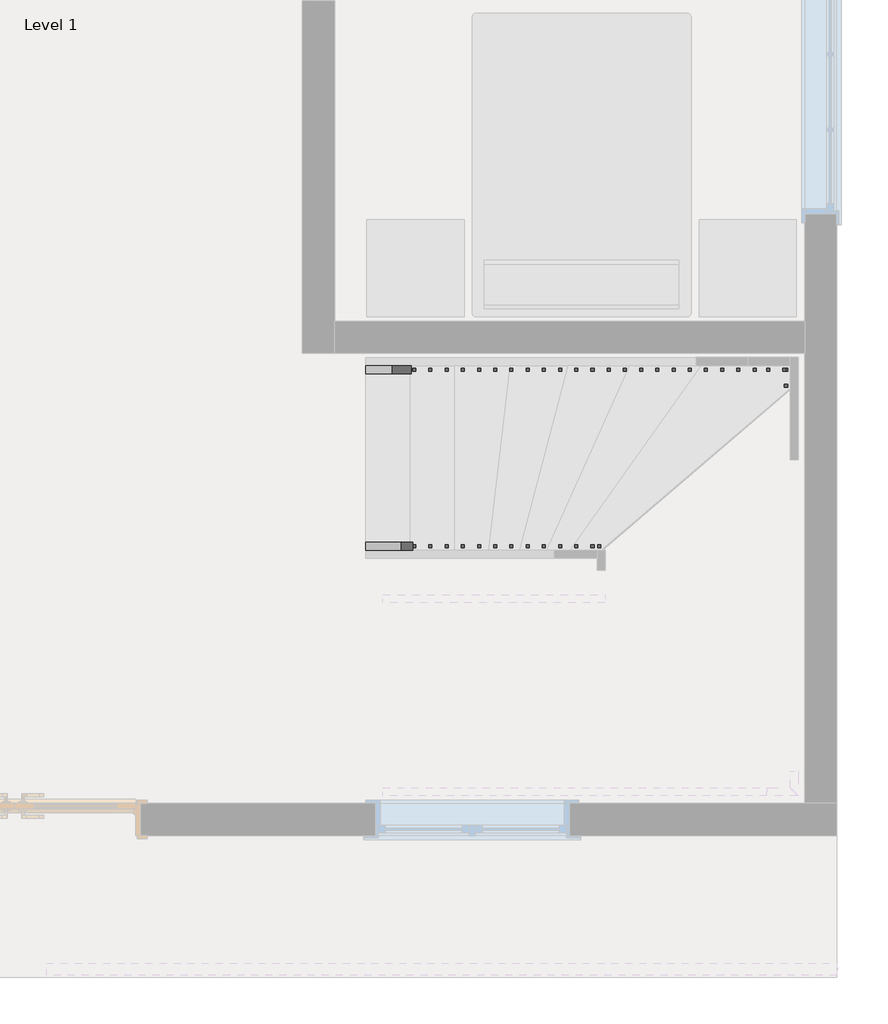
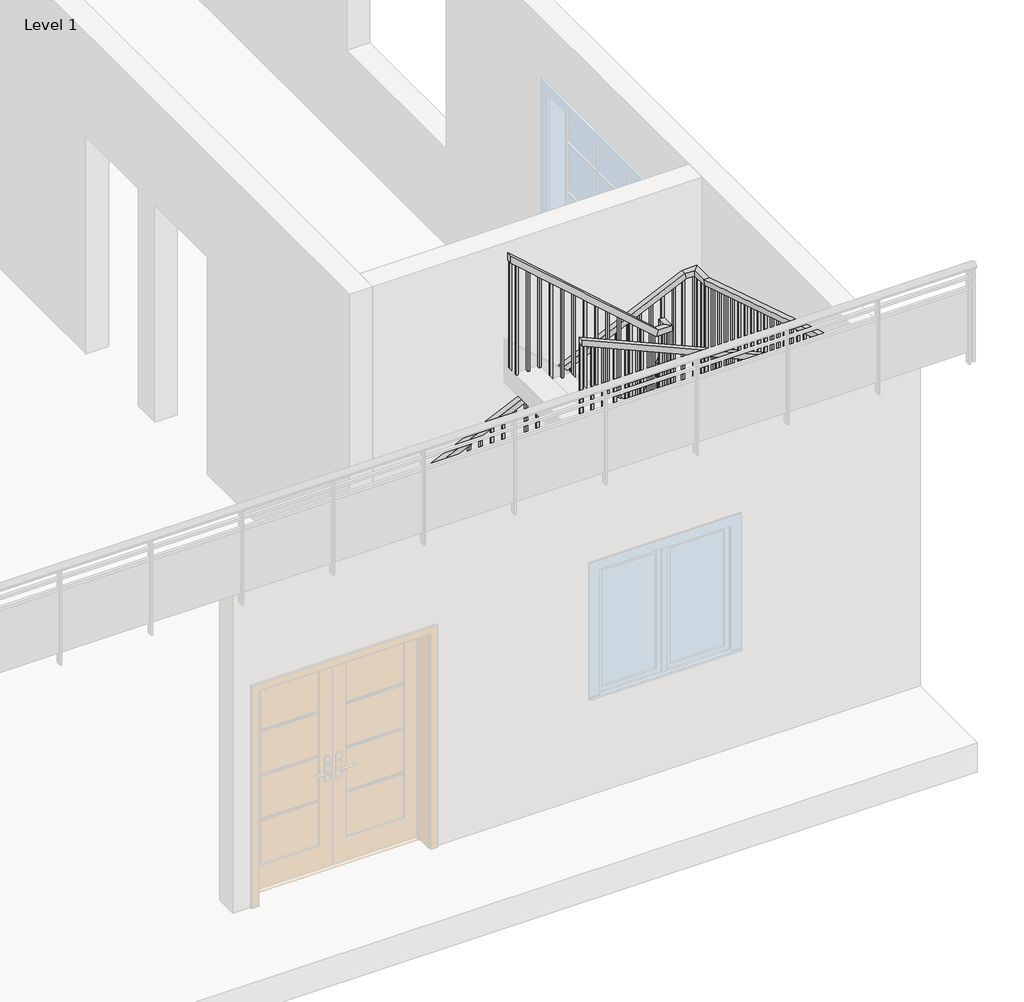
# One storey, part 3 of 4: 2 railings.
"""IFC4 building model written with IfcOpenShell, lengths in millimetres."""

from ifc_helpers import new_model, si_unit, frame, origin, place, context, project, spatial, polyline, outline, extrude, faceted_brep, element, save

model = new_model("IFC4")

# Units and contexts
model_context = context("Model", 3, world=origin())
ifc_project = project(units=[si_unit("LENGTHUNIT", "METRE", prefix="MILLI")], contexts=[model_context])

# Site, building, storey
site = spatial("IfcSite", under=ifc_project)
building = spatial("IfcBuilding", under=site)
storey = spatial("IfcBuildingStorey", under=building, Name="Level 1", Elevation=0.0)

# Railings
placement = place(None, origin())
element("IfcRailing", 1, ObjectType="Handrail - Rectangular", at=placement, inside=storey, context=model_context, shape_type="SolidModel", body=[
    faceted_brep([(-5318.5510787, 1481.9501077, 1007.9778391), (-5318.5510787, 1481.9501077, 940.4028685), (-5318.5510787, 1431.1501077, 940.4028685), (-5318.5510787, 1431.1501077, 1007.9778391), (-3853.6690894, 1481.9501077, 2292.967851), (-3834.5457095, 1481.9501077, 2242.167851), (-3834.5457095, 1431.1501077, 2242.167851), (-3853.6690894, 1431.1501077, 2292.967851), (-3764.9367614, 1481.9501077, 2292.967851), (-3764.9367614, 1431.1501077, 2292.967851), (-3764.9367614, 1431.1501077, 2242.167851), (-3764.9367614, 1481.9501077, 2242.167851)], [[[0, 1, 2, 3]], [[1, 0, 4, 5]], [[2, 1, 5, 6]], [[3, 2, 6, 7]], [[0, 3, 7, 4]], [[8, 9, 10, 11]], [[5, 4, 8, 11]], [[6, 5, 11, 10]], [[7, 6, 10, 9]], [[4, 7, 9, 8]]]),
    faceted_brep([(-3764.9367614, 1431.1501077, 2288.9786494), (-3764.9367614, 1431.1501077, 2174.0145886), (-3815.7367614, 1431.1501077, 2174.0145886), (-3815.7367614, 1431.1501077, 2288.9786494), (-3764.9367614, 1177.1501077, 2804.6358827), (-3764.9367614, 1126.3501077, 2792.8032685), (-3815.7367614, 1126.3501077, 2792.8032685), (-3815.7367614, 1177.1501077, 2804.6358827), (-5209.7542153, 1050.1501077, 4209.1766651), (-5209.7542153, 1100.9501077, 4209.1766651), (-5209.7542153, 1100.9501077, 4141.3989335), (-5209.7542153, 1050.1501077, 4141.3989335), (-3911.1589121, 1050.1501077, 2994.4303641), (-3891.9367614, 1050.1501077, 3045.2303641), (-3911.1589121, 1100.9501077, 2994.4303641), (-3891.9367614, 1100.9501077, 3045.2303641), (-3764.9367614, 1177.1501077, 3045.2303641), (-3764.9367614, 1126.3501077, 2994.4303641), (-3815.7367614, 1126.3501077, 2994.4303641), (-3815.7367614, 1177.1501077, 3045.2303641), (-3764.9367614, 1050.1501077, 3045.2303641), (-3764.9367614, 1050.1501077, 2994.4303641), (-3815.7367614, 1100.9501077, 2994.4303641), (-3815.7367614, 1100.9501077, 3045.2303641)], [[[0, 1, 2, 3]], [[1, 0, 4, 5]], [[2, 1, 5, 6]], [[3, 2, 6, 7]], [[0, 3, 7, 4]], [[8, 9, 10, 11]], [[12, 13, 8, 11]], [[14, 12, 11, 10]], [[15, 14, 10, 9]], [[13, 15, 9, 8]], [[5, 4, 16, 17]], [[6, 5, 17, 18]], [[7, 6, 18, 19]], [[4, 7, 19, 16]], [[17, 16, 20, 21]], [[18, 17, 21, 22]], [[19, 18, 22, 23]], [[16, 19, 23, 20]], [[21, 20, 13, 12]], [[22, 21, 12, 14]], [[23, 22, 14, 15]], [[20, 23, 15, 13]]]),
    extrude(outline(polyline([(4073.5861118, -5132.976687), (4090.4117935, -5152.026687), (3048.0, -5152.026687), (3048.0, -5132.976687), (4073.5861118, -5132.976687)])), frame((0.0, 1066.0251077, 0.0), z_axis=(0.0, 1.0, 0.0), x_axis=(0.0, 0.0, 1.0)), (0.0, 0.0, 1.0), 19.05),
    extrude(outline(polyline([(3983.8491427, -5031.376687), (4000.6748244, -5050.426687), (3048.0, -5050.426687), (3048.0, -5031.376687), (3983.8491427, -5031.376687)])), frame((0.0, 1066.0251077, 0.0), z_axis=(0.0, 1.0, 0.0), x_axis=(0.0, 0.0, 1.0)), (0.0, 0.0, 1.0), 19.05),
    extrude(outline(polyline([(3894.1121735, -4929.776687), (3910.9378552, -4948.826687), (3048.0, -4948.826687), (3048.0, -4929.776687), (3894.1121735, -4929.776687)])), frame((0.0, 1066.0251077, 0.0), z_axis=(0.0, 1.0, 0.0), x_axis=(0.0, 0.0, 1.0)), (0.0, 0.0, 1.0), 19.05),
    extrude(outline(polyline([(3804.3752044, -4828.176687), (3821.2008861, -4847.226687), (2878.6666667, -4847.226687), (2878.6666667, -4828.176687), (3804.3752044, -4828.176687)])), frame((0.0, 1066.0251077, 0.0), z_axis=(0.0, 1.0, 0.0), x_axis=(0.0, 0.0, 1.0)), (0.0, 0.0, 1.0), 19.05),
    extrude(outline(polyline([(3714.6382352, -4726.576687), (3731.4639169, -4745.626687), (2878.6666667, -4745.626687), (2878.6666667, -4726.576687), (3714.6382352, -4726.576687)])), frame((0.0, 1066.0251077, 0.0), z_axis=(0.0, 1.0, 0.0), x_axis=(0.0, 0.0, 1.0)), (0.0, 0.0, 1.0), 19.05),
    extrude(outline(polyline([(3624.9012661, -4624.976687), (3641.7269478, -4644.026687), (2709.3333333, -4644.026687), (2709.3333333, -4624.976687), (3624.9012661, -4624.976687)])), frame((0.0, 1066.0251077, 0.0), z_axis=(0.0, 1.0, 0.0), x_axis=(0.0, 0.0, 1.0)), (0.0, 0.0, 1.0), 19.05),
    extrude(outline(polyline([(3535.1642969, -4523.376687), (3551.9899786, -4542.426687), (2709.3333333, -4542.426687), (2709.3333333, -4523.376687), (3535.1642969, -4523.376687)])), frame((0.0, 1066.0251077, 0.0), z_axis=(0.0, 1.0, 0.0), x_axis=(0.0, 0.0, 1.0)), (0.0, 0.0, 1.0), 19.05),
    extrude(outline(polyline([(3445.4273278, -4421.776687), (3462.2530095, -4440.826687), (2540.0, -4440.826687), (2540.0, -4421.776687), (3445.4273278, -4421.776687)])), frame((0.0, 1066.0251077, 0.0), z_axis=(0.0, 1.0, 0.0), x_axis=(0.0, 0.0, 1.0)), (0.0, 0.0, 1.0), 19.05),
    extrude(outline(polyline([(3355.6903586, -4320.176687), (3372.5160404, -4339.226687), (2540.0, -4339.226687), (2540.0, -4320.176687), (3355.6903586, -4320.176687)])), frame((0.0, 1066.0251077, 0.0), z_axis=(0.0, 1.0, 0.0), x_axis=(0.0, 0.0, 1.0)), (0.0, 0.0, 1.0), 19.05),
    extrude(outline(polyline([(3265.9533895, -4218.576687), (3282.7790712, -4237.626687), (2370.6666667, -4237.626687), (2370.6666667, -4218.576687), (3265.9533895, -4218.576687)])), frame((0.0, 1066.0251077, 0.0), z_axis=(0.0, 1.0, 0.0), x_axis=(0.0, 0.0, 1.0)), (0.0, 0.0, 1.0), 19.05),
    extrude(outline(polyline([(3176.2164204, -4116.976687), (3193.0421021, -4136.026687), (2370.6666667, -4136.026687), (2370.6666667, -4116.976687), (3176.2164204, -4116.976687)])), frame((0.0, 1066.0251077, 0.0), z_axis=(0.0, 1.0, 0.0), x_axis=(0.0, 0.0, 1.0)), (0.0, 0.0, 1.0), 19.05),
    extrude(outline(polyline([(3086.4794512, -4015.376687), (3103.3051329, -4034.426687), (2201.3333333, -4034.426687), (2201.3333333, -4015.376687), (3086.4794512, -4015.376687)])), frame((0.0, 1066.0251077, 0.0), z_axis=(0.0, 1.0, 0.0), x_axis=(0.0, 0.0, 1.0)), (0.0, 0.0, 1.0), 19.05),
    extrude(outline(polyline([(2996.7424821, -3913.776687), (3013.5681638, -3932.826687), (2032.0, -3932.826687), (2032.0, -3913.776687), (2996.7424821, -3913.776687)])), frame((0.0, 1066.0251077, 0.0), z_axis=(0.0, 1.0, 0.0), x_axis=(0.0, 0.0, 1.0)), (0.0, 0.0, 1.0), 19.05),
    extrude(outline(polyline([(1114.8601257, 2816.1296163), (1133.9101257, 2777.4553238), (1133.9101257, 1862.6666667), (1114.8601257, 1862.6666667), (1114.8601257, 2816.1296163)])), frame((-3799.8617614, 0.0, 0.0), z_axis=(1.0, 0.0, 0.0), x_axis=(0.0, 1.0, 0.0)), (0.0, 0.0, 1.0), 19.05),
    extrude(outline(polyline([(1216.4601257, 2609.866723), (1235.5101257, 2571.1924305), (1235.5101257, 1693.3333333), (1216.4601257, 1693.3333333), (1216.4601257, 2609.866723)])), frame((-3799.8617614, 0.0, 0.0), z_axis=(1.0, 0.0, 0.0), x_axis=(0.0, 1.0, 0.0)), (0.0, 0.0, 1.0), 19.05),
    extrude(outline(polyline([(1318.0601257, 2403.6038297), (1337.1101257, 2364.9295372), (1337.1101257, 1524.0), (1318.0601257, 1524.0), (1318.0601257, 2403.6038297)])), frame((-3799.8617614, 0.0, 0.0), z_axis=(1.0, 0.0, 0.0), x_axis=(0.0, 1.0, 0.0)), (0.0, 0.0, 1.0), 19.05),
    extrude(outline(polyline([(2196.48311, -3886.6260787), (2179.7725081, -3905.6760787), (1185.3333333, -3905.6760787), (1185.3333333, -3886.6260787), (2196.48311, -3886.6260787)])), frame((0.0, 1447.0251077, 0.0), z_axis=(0.0, 1.0, 0.0), x_axis=(0.0, 0.0, 1.0)), (0.0, 0.0, 1.0), 19.05),
    extrude(outline(polyline([(2107.3598999, -3988.2260787), (2090.6492981, -4007.2760787), (1185.3333333, -4007.2760787), (1185.3333333, -3988.2260787), (2107.3598999, -3988.2260787)])), frame((0.0, 1447.0251077, 0.0), z_axis=(0.0, 1.0, 0.0), x_axis=(0.0, 0.0, 1.0)), (0.0, 0.0, 1.0), 19.05),
    extrude(outline(polyline([(2018.2366899, -4089.8260787), (2001.526088, -4108.8760787), (1016.0, -4108.8760787), (1016.0, -4089.8260787), (2018.2366899, -4089.8260787)])), frame((0.0, 1447.0251077, 0.0), z_axis=(0.0, 1.0, 0.0), x_axis=(0.0, 0.0, 1.0)), (0.0, 0.0, 1.0), 19.05),
    extrude(outline(polyline([(1929.1134799, -4191.4260787), (1912.402878, -4210.4760787), (846.6666667, -4210.4760787), (846.6666667, -4191.4260787), (1929.1134799, -4191.4260787)])), frame((0.0, 1447.0251077, 0.0), z_axis=(0.0, 1.0, 0.0), x_axis=(0.0, 0.0, 1.0)), (0.0, 0.0, 1.0), 19.05),
    extrude(outline(polyline([(1839.9902698, -4293.0260787), (1823.279668, -4312.0760787), (846.6666667, -4312.0760787), (846.6666667, -4293.0260787), (1839.9902698, -4293.0260787)])), frame((0.0, 1447.0251077, 0.0), z_axis=(0.0, 1.0, 0.0), x_axis=(0.0, 0.0, 1.0)), (0.0, 0.0, 1.0), 19.05),
    extrude(outline(polyline([(1750.8670598, -4394.6260787), (1734.1564579, -4413.6760787), (677.3333333, -4413.6760787), (677.3333333, -4394.6260787), (1750.8670598, -4394.6260787)])), frame((0.0, 1447.0251077, 0.0), z_axis=(0.0, 1.0, 0.0), x_axis=(0.0, 0.0, 1.0)), (0.0, 0.0, 1.0), 19.05),
    extrude(outline(polyline([(1661.7438498, -4496.2260787), (1645.0332479, -4515.2760787), (677.3333333, -4515.2760787), (677.3333333, -4496.2260787), (1661.7438498, -4496.2260787)])), frame((0.0, 1447.0251077, 0.0), z_axis=(0.0, 1.0, 0.0), x_axis=(0.0, 0.0, 1.0)), (0.0, 0.0, 1.0), 19.05),
    extrude(outline(polyline([(1572.6206397, -4597.8260787), (1555.9100378, -4616.8760787), (508.0, -4616.8760787), (508.0, -4597.8260787), (1572.6206397, -4597.8260787)])), frame((0.0, 1447.0251077, 0.0), z_axis=(0.0, 1.0, 0.0), x_axis=(0.0, 0.0, 1.0)), (0.0, 0.0, 1.0), 19.05),
    extrude(outline(polyline([(1483.4974297, -4699.4260787), (1466.7868278, -4718.4760787), (508.0, -4718.4760787), (508.0, -4699.4260787), (1483.4974297, -4699.4260787)])), frame((0.0, 1447.0251077, 0.0), z_axis=(0.0, 1.0, 0.0), x_axis=(0.0, 0.0, 1.0)), (0.0, 0.0, 1.0), 19.05),
    extrude(outline(polyline([(1394.3742197, -4801.0260787), (1377.6636178, -4820.0760787), (338.6666667, -4820.0760787), (338.6666667, -4801.0260787), (1394.3742197, -4801.0260787)])), frame((0.0, 1447.0251077, 0.0), z_axis=(0.0, 1.0, 0.0), x_axis=(0.0, 0.0, 1.0)), (0.0, 0.0, 1.0), 19.05),
    extrude(outline(polyline([(1305.2510096, -4902.6260787), (1288.5404077, -4921.6760787), (338.6666667, -4921.6760787), (338.6666667, -4902.6260787), (1305.2510096, -4902.6260787)])), frame((0.0, 1447.0251077, 0.0), z_axis=(0.0, 1.0, 0.0), x_axis=(0.0, 0.0, 1.0)), (0.0, 0.0, 1.0), 19.05),
    extrude(outline(polyline([(1216.1277996, -5004.2260787), (1199.4171977, -5023.2760787), (338.6666667, -5023.2760787), (338.6666667, -5004.2260787), (1216.1277996, -5004.2260787)])), frame((0.0, 1447.0251077, 0.0), z_axis=(0.0, 1.0, 0.0), x_axis=(0.0, 0.0, 1.0)), (0.0, 0.0, 1.0), 19.05),
    extrude(outline(polyline([(1127.0045896, -5105.8260787), (1110.2939877, -5124.8760787), (169.3333333, -5124.8760787), (169.3333333, -5105.8260787), (1127.0045896, -5105.8260787)])), frame((0.0, 1447.0251077, 0.0), z_axis=(0.0, 1.0, 0.0), x_axis=(0.0, 0.0, 1.0)), (0.0, 0.0, 1.0), 19.05),
    extrude(outline(polyline([(1037.8813795, -5207.4260787), (1021.1707776, -5226.4760787), (169.3333333, -5226.4760787), (169.3333333, -5207.4260787), (1037.8813795, -5207.4260787)])), frame((0.0, 1447.0251077, 0.0), z_axis=(0.0, 1.0, 0.0), x_axis=(0.0, 0.0, 1.0)), (0.0, 0.0, 1.0), 19.05),
    extrude(outline(polyline([(-3812.176687, 1085.0751077), (-3812.176687, 1066.0251077), (-3831.226687, 1066.0251077), (-3831.226687, 1085.0751077), (-3812.176687, 1085.0751077)])), frame((0.0, 0.0, 2032.0), z_axis=(0.0, 0.0, 1.0), x_axis=(1.0, 0.0, 0.0)), (0.0, 0.0, 1.0), 962.4303641),
    extrude(outline(polyline([(-3799.8617614, 1085.0751077), (-3780.8117614, 1085.0751077), (-3780.8117614, 1066.0251077), (-3799.8617614, 1066.0251077), (-3799.8617614, 1085.0751077)])), frame((0.0, 0.0, 2032.0), z_axis=(0.0, 0.0, 1.0), x_axis=(1.0, 0.0, 0.0)), (0.0, 0.0, 1.0), 962.4303641),
    extrude(outline(polyline([(-3799.8617614, 1098.7207679), (-3780.8117614, 1098.7207679), (-3780.8117614, 1079.6707679), (-3799.8617614, 1079.6707679), (-3799.8617614, 1098.7207679)])), frame((0.0, 0.0, 2032.0), z_axis=(0.0, 0.0, 1.0), x_axis=(1.0, 0.0, 0.0)), (0.0, 0.0, 1.0), 962.4303641),
    extrude(outline(polyline([(1419.6601257, 2197.3409364), (1438.7101257, 2158.6666439), (1438.7101257, 1354.6666667), (1419.6601257, 1354.6666667), (1419.6601257, 2197.3409364)])), frame((-3799.8617614, 0.0, 0.0), z_axis=(1.0, 0.0, 0.0), x_axis=(0.0, 1.0, 0.0)), (0.0, 0.0, 1.0), 19.05),
    extrude(outline(polyline([(-3799.8617614, 1447.0251077), (-3799.8617614, 1466.0751077), (-3780.8117614, 1466.0751077), (-3780.8117614, 1447.0251077), (-3799.8617614, 1447.0251077)])), frame((0.0, 0.0, 1354.6666667), z_axis=(0.0, 0.0, 1.0), x_axis=(1.0, 0.0, 0.0)), (0.0, 0.0, 1.0), 887.5011843),
    extrude(outline(polyline([(2233.7481814, -3844.1440894), (2217.0375795, -3863.1940894), (1185.3333333, -3863.1940894), (1185.3333333, -3844.1440894), (2233.7481814, -3844.1440894)])), frame((0.0, 1447.0251077, 0.0), z_axis=(0.0, 1.0, 0.0), x_axis=(0.0, 0.0, 1.0)), (0.0, 0.0, 1.0), 19.05),
    extrude(outline(polyline([(4124.5732518, -5190.7042153), (4141.3989335, -5209.7542153), (3048.0, -5209.7542153), (3048.0, -5190.7042153), (4124.5732518, -5190.7042153)])), frame((0.0, 1066.0251077, 0.0), z_axis=(0.0, 1.0, 0.0), x_axis=(0.0, 0.0, 1.0)), (0.0, 0.0, 1.0), 19.05),
    extrude(outline(polyline([(957.1134704, -5299.5010787), (940.4028685, -5318.5510787), (169.3333333, -5318.5510787), (169.3333333, -5299.5010787), (957.1134704, -5299.5010787)])), frame((0.0, 1447.0251077, 0.0), z_axis=(0.0, 1.0, 0.0), x_axis=(0.0, 0.0, 1.0)), (0.0, 0.0, 1.0), 19.05),
])
element("IfcRailing", 2, ObjectType="Handrail - Rectangular", at=placement, inside=storey, context=model_context, shape_type="SolidModel", body=[
    faceted_brep([(-5318.5510787, 2589.1174997, 1123.4764008), (-5318.5510787, 2589.1174997, 1067.4781727), (-5318.5510787, 2538.3174997, 1067.4781727), (-5318.5510787, 2538.3174997, 1123.4764008), (-2794.8351304, 2589.1174997, 2294.0169189), (-2783.6276147, 2589.1174997, 2243.2169189), (-2783.6276147, 2538.3174997, 2243.2169189), (-2794.8351304, 2538.3174997, 2294.0169189), (-2657.7693695, 2589.1174997, 2294.0169189), (-2657.7693695, 2589.1174997, 2243.2169189), (-2708.5693695, 2538.3174997, 2243.2169189), (-2708.5693695, 2538.3174997, 2294.0169189), (-2657.7693695, 2398.3356848, 2294.0169189), (-2657.7693695, 2390.5672195, 2243.2169189), (-2708.5693695, 2390.5672195, 2243.2169189), (-2708.5693695, 2398.3356848, 2294.0169189), (-2657.7693695, -57.0172843, 2966.0525983), (-2657.7693695, -57.0172843, 3016.8525983), (-2770.3188697, -57.0172843, 3016.8525983), (-2780.9506148, -57.0172843, 2966.0525983), (-2708.5693695, -6.2172843, 2966.0525983), (-2780.9506148, -6.2172843, 2966.0525983), (-2708.5693695, -6.2172843, 3016.8525983), (-2770.3188697, -6.2172843, 3016.8525983), (-2657.7693695, 90.2000505, 3016.8525983), (-2657.7693695, 82.4315853, 2966.0525983), (-2708.5693695, 82.4315853, 2966.0525983), (-2708.5693695, 90.2000505, 3016.8525983), (-5209.7542153, -57.0172843, 4084.706306), (-5209.7542153, -6.2172843, 4084.706306), (-5209.7542153, -6.2172843, 4029.2522993), (-5209.7542153, -57.0172843, 4029.2522993)], [[[0, 1, 2, 3]], [[1, 0, 4, 5]], [[2, 1, 5, 6]], [[3, 2, 6, 7]], [[0, 3, 7, 4]], [[5, 4, 8, 9]], [[6, 5, 9, 10]], [[7, 6, 10, 11]], [[4, 7, 11, 8]], [[9, 8, 12, 13]], [[10, 9, 13, 14]], [[11, 10, 14, 15]], [[8, 11, 15, 12]], [[16, 17, 18, 19]], [[20, 16, 19, 21]], [[22, 20, 21, 23]], [[17, 22, 23, 18]], [[13, 12, 24, 25]], [[14, 13, 25, 26]], [[15, 14, 26, 27]], [[12, 15, 27, 24]], [[25, 24, 17, 16]], [[26, 25, 16, 20]], [[27, 26, 20, 22]], [[24, 27, 22, 17]], [[28, 29, 30, 31]], [[19, 18, 28, 31]], [[21, 19, 31, 30]], [[23, 21, 30, 29]], [[18, 23, 29, 28]]]),
    extrude(outline(polyline([(4032.9686139, -5218.2438697), (3048.0, -5218.2438697), (3048.0, -5199.1938697), (4024.6295475, -5199.1938697), (4032.9686139, -5218.2438697)])), frame((0.0, -41.1422843, 0.0), z_axis=(0.0, 1.0, 0.0), x_axis=(0.0, 0.0, 1.0)), (0.0, 0.0, 1.0), 19.05),
    extrude(outline(polyline([(3988.4935935, -5116.6438697), (3048.0, -5116.6438697), (3048.0, -5097.5938697), (3980.1545272, -5097.5938697), (3988.4935935, -5116.6438697)])), frame((0.0, -41.1422843, 0.0), z_axis=(0.0, 1.0, 0.0), x_axis=(0.0, 0.0, 1.0)), (0.0, 0.0, 1.0), 19.05),
    extrude(outline(polyline([(3944.0185731, -5015.0438697), (3048.0, -5015.0438697), (3048.0, -4995.9938697), (3935.6795068, -4995.9938697), (3944.0185731, -5015.0438697)])), frame((0.0, -41.1422843, 0.0), z_axis=(0.0, 1.0, 0.0), x_axis=(0.0, 0.0, 1.0)), (0.0, 0.0, 1.0), 19.05),
    extrude(outline(polyline([(3899.5435527, -4913.4438697), (2878.6666667, -4913.4438697), (2878.6666667, -4894.3938697), (3891.2044864, -4894.3938697), (3899.5435527, -4913.4438697)])), frame((0.0, -41.1422843, 0.0), z_axis=(0.0, 1.0, 0.0), x_axis=(0.0, 0.0, 1.0)), (0.0, 0.0, 1.0), 19.05),
    extrude(outline(polyline([(3855.0685323, -4811.8438697), (2878.6666667, -4811.8438697), (2878.6666667, -4792.7938697), (3846.729466, -4792.7938697), (3855.0685323, -4811.8438697)])), frame((0.0, -41.1422843, 0.0), z_axis=(0.0, 1.0, 0.0), x_axis=(0.0, 0.0, 1.0)), (0.0, 0.0, 1.0), 19.05),
    extrude(outline(polyline([(3810.593512, -4710.2438697), (2878.6666667, -4710.2438697), (2878.6666667, -4691.1938697), (3802.2544456, -4691.1938697), (3810.593512, -4710.2438697)])), frame((0.0, -41.1422843, 0.0), z_axis=(0.0, 1.0, 0.0), x_axis=(0.0, 0.0, 1.0)), (0.0, 0.0, 1.0), 19.05),
    extrude(outline(polyline([(3766.1184916, -4608.6438697), (2709.3333333, -4608.6438697), (2709.3333333, -4589.5938697), (3757.7794253, -4589.5938697), (3766.1184916, -4608.6438697)])), frame((0.0, -41.1422843, 0.0), z_axis=(0.0, 1.0, 0.0), x_axis=(0.0, 0.0, 1.0)), (0.0, 0.0, 1.0), 19.05),
    extrude(outline(polyline([(3721.6434712, -4507.0438697), (2709.3333333, -4507.0438697), (2709.3333333, -4487.9938697), (3713.3044049, -4487.9938697), (3721.6434712, -4507.0438697)])), frame((0.0, -41.1422843, 0.0), z_axis=(0.0, 1.0, 0.0), x_axis=(0.0, 0.0, 1.0)), (0.0, 0.0, 1.0), 19.05),
    extrude(outline(polyline([(3677.1684508, -4405.4438697), (2709.3333333, -4405.4438697), (2709.3333333, -4386.3938697), (3668.8293845, -4386.3938697), (3677.1684508, -4405.4438697)])), frame((0.0, -41.1422843, 0.0), z_axis=(0.0, 1.0, 0.0), x_axis=(0.0, 0.0, 1.0)), (0.0, 0.0, 1.0), 19.05),
    extrude(outline(polyline([(3632.6934304, -4303.8438697), (2540.0, -4303.8438697), (2540.0, -4284.7938697), (3624.3543641, -4284.7938697), (3632.6934304, -4303.8438697)])), frame((0.0, -41.1422843, 0.0), z_axis=(0.0, 1.0, 0.0), x_axis=(0.0, 0.0, 1.0)), (0.0, 0.0, 1.0), 19.05),
    extrude(outline(polyline([(3588.2184101, -4202.2438697), (2540.0, -4202.2438697), (2540.0, -4183.1938697), (3579.8793437, -4183.1938697), (3588.2184101, -4202.2438697)])), frame((0.0, -41.1422843, 0.0), z_axis=(0.0, 1.0, 0.0), x_axis=(0.0, 0.0, 1.0)), (0.0, 0.0, 1.0), 19.05),
    extrude(outline(polyline([(3543.7433897, -4100.6438697), (2540.0, -4100.6438697), (2540.0, -4081.5938697), (3535.4043233, -4081.5938697), (3543.7433897, -4100.6438697)])), frame((0.0, -41.1422843, 0.0), z_axis=(0.0, 1.0, 0.0), x_axis=(0.0, 0.0, 1.0)), (0.0, 0.0, 1.0), 19.05),
    extrude(outline(polyline([(3499.2683693, -3999.0438697), (2540.0, -3999.0438697), (2540.0, -3979.9938697), (3490.929303, -3979.9938697), (3499.2683693, -3999.0438697)])), frame((0.0, -41.1422843, 0.0), z_axis=(0.0, 1.0, 0.0), x_axis=(0.0, 0.0, 1.0)), (0.0, 0.0, 1.0), 19.05),
    extrude(outline(polyline([(3454.7933489, -3897.4438697), (2370.6666667, -3897.4438697), (2370.6666667, -3878.3938697), (3446.4542826, -3878.3938697), (3454.7933489, -3897.4438697)])), frame((0.0, -41.1422843, 0.0), z_axis=(0.0, 1.0, 0.0), x_axis=(0.0, 0.0, 1.0)), (0.0, 0.0, 1.0), 19.05),
    extrude(outline(polyline([(3410.3183285, -3795.8438697), (2370.6666667, -3795.8438697), (2370.6666667, -3776.7938697), (3401.9792622, -3776.7938697), (3410.3183285, -3795.8438697)])), frame((0.0, -41.1422843, 0.0), z_axis=(0.0, 1.0, 0.0), x_axis=(0.0, 0.0, 1.0)), (0.0, 0.0, 1.0), 19.05),
    extrude(outline(polyline([(3365.8433081, -3694.2438697), (2370.6666667, -3694.2438697), (2370.6666667, -3675.1938697), (3357.5042418, -3675.1938697), (3365.8433081, -3694.2438697)])), frame((0.0, -41.1422843, 0.0), z_axis=(0.0, 1.0, 0.0), x_axis=(0.0, 0.0, 1.0)), (0.0, 0.0, 1.0), 19.05),
    extrude(outline(polyline([(3321.3682878, -3592.6438697), (2370.6666667, -3592.6438697), (2370.6666667, -3573.5938697), (3313.0292214, -3573.5938697), (3321.3682878, -3592.6438697)])), frame((0.0, -41.1422843, 0.0), z_axis=(0.0, 1.0, 0.0), x_axis=(0.0, 0.0, 1.0)), (0.0, 0.0, 1.0), 19.05),
    extrude(outline(polyline([(3276.8932674, -3491.0438697), (2201.3333333, -3491.0438697), (2201.3333333, -3471.9938697), (3268.5542011, -3471.9938697), (3276.8932674, -3491.0438697)])), frame((0.0, -41.1422843, 0.0), z_axis=(0.0, 1.0, 0.0), x_axis=(0.0, 0.0, 1.0)), (0.0, 0.0, 1.0), 19.05),
    extrude(outline(polyline([(3232.418247, -3389.4438697), (2201.3333333, -3389.4438697), (2201.3333333, -3370.3938697), (3224.0791807, -3370.3938697), (3232.418247, -3389.4438697)])), frame((0.0, -41.1422843, 0.0), z_axis=(0.0, 1.0, 0.0), x_axis=(0.0, 0.0, 1.0)), (0.0, 0.0, 1.0), 19.05),
    extrude(outline(polyline([(3187.9432266, -3287.8438697), (2201.3333333, -3287.8438697), (2201.3333333, -3268.7938697), (3179.6041603, -3268.7938697), (3187.9432266, -3287.8438697)])), frame((0.0, -41.1422843, 0.0), z_axis=(0.0, 1.0, 0.0), x_axis=(0.0, 0.0, 1.0)), (0.0, 0.0, 1.0), 19.05),
    extrude(outline(polyline([(3143.4682062, -3186.2438697), (2201.3333333, -3186.2438697), (2201.3333333, -3167.1938697), (3135.1291399, -3167.1938697), (3143.4682062, -3186.2438697)])), frame((0.0, -41.1422843, 0.0), z_axis=(0.0, 1.0, 0.0), x_axis=(0.0, 0.0, 1.0)), (0.0, 0.0, 1.0), 19.05),
    extrude(outline(polyline([(3098.9931859, -3084.6438697), (2201.3333333, -3084.6438697), (2201.3333333, -3065.5938697), (3090.6541195, -3065.5938697), (3098.9931859, -3084.6438697)])), frame((0.0, -41.1422843, 0.0), z_axis=(0.0, 1.0, 0.0), x_axis=(0.0, 0.0, 1.0)), (0.0, 0.0, 1.0), 19.05),
    extrude(outline(polyline([(3054.5181655, -2983.0438697), (2032.0, -2983.0438697), (2032.0, -2963.9938697), (3046.1790992, -2963.9938697), (3054.5181655, -2983.0438697)])), frame((0.0, -41.1422843, 0.0), z_axis=(0.0, 1.0, 0.0), x_axis=(0.0, 0.0, 1.0)), (0.0, 0.0, 1.0), 19.05),
    extrude(outline(polyline([(3010.0431451, -2881.4438697), (2032.0, -2881.4438697), (2032.0, -2862.3938697), (3001.7040788, -2862.3938697), (3010.0431451, -2881.4438697)])), frame((0.0, -41.1422843, 0.0), z_axis=(0.0, 1.0, 0.0), x_axis=(0.0, 0.0, 1.0)), (0.0, 0.0, 1.0), 19.05),
    extrude(outline(polyline([(-2673.6443695, -1.8749495), (-2673.6443695, -20.9249495), (-2692.6943695, -20.9249495), (-2692.6943695, -1.8749495), (-2673.6443695, -1.8749495)])), frame((0.0, 0.0, 2032.0), z_axis=(0.0, 0.0, 1.0), x_axis=(1.0, 0.0, 0.0)), (0.0, 0.0, 1.0), 934.0525983),
    extrude(outline(polyline([(172.6606848, 2937.7956746), (172.6606848, 2032.0), (153.6106848, 2032.0), (153.6106848, 2943.761537), (172.6606848, 2937.7956746)])), frame((-2692.6943695, 0.0, 0.0), z_axis=(1.0, 0.0, 0.0), x_axis=(0.0, 1.0, 0.0)), (0.0, 0.0, 1.0), 19.05),
    extrude(outline(polyline([(274.2606848, 2905.9777416), (274.2606848, 2032.0), (255.2106848, 2032.0), (255.2106848, 2911.943604), (274.2606848, 2905.9777416)])), frame((-2692.6943695, 0.0, 0.0), z_axis=(1.0, 0.0, 0.0), x_axis=(0.0, 1.0, 0.0)), (0.0, 0.0, 1.0), 19.05),
    extrude(outline(polyline([(375.8606848, 2874.1598085), (375.8606848, 1862.6666667), (356.8106848, 1862.6666667), (356.8106848, 2880.125671), (375.8606848, 2874.1598085)])), frame((-2692.6943695, 0.0, 0.0), z_axis=(1.0, 0.0, 0.0), x_axis=(0.0, 1.0, 0.0)), (0.0, 0.0, 1.0), 19.05),
    extrude(outline(polyline([(477.4606848, 2842.3418755), (477.4606848, 1862.6666667), (458.4106848, 1862.6666667), (458.4106848, 2848.3077379), (477.4606848, 2842.3418755)])), frame((-2692.6943695, 0.0, 0.0), z_axis=(1.0, 0.0, 0.0), x_axis=(0.0, 1.0, 0.0)), (0.0, 0.0, 1.0), 19.05),
    extrude(outline(polyline([(579.0606848, 2810.5239425), (579.0606848, 1862.6666667), (560.0106848, 1862.6666667), (560.0106848, 2816.4898049), (579.0606848, 2810.5239425)])), frame((-2692.6943695, 0.0, 0.0), z_axis=(1.0, 0.0, 0.0), x_axis=(0.0, 1.0, 0.0)), (0.0, 0.0, 1.0), 19.05),
    extrude(outline(polyline([(680.6606848, 2778.7060094), (680.6606848, 1862.6666667), (661.6106848, 1862.6666667), (661.6106848, 2784.6718719), (680.6606848, 2778.7060094)])), frame((-2692.6943695, 0.0, 0.0), z_axis=(1.0, 0.0, 0.0), x_axis=(0.0, 1.0, 0.0)), (0.0, 0.0, 1.0), 19.05),
    extrude(outline(polyline([(782.2606848, 2746.8880764), (782.2606848, 1862.6666667), (763.2106848, 1862.6666667), (763.2106848, 2752.8539389), (782.2606848, 2746.8880764)])), frame((-2692.6943695, 0.0, 0.0), z_axis=(1.0, 0.0, 0.0), x_axis=(0.0, 1.0, 0.0)), (0.0, 0.0, 1.0), 19.05),
    extrude(outline(polyline([(883.8606848, 2715.0701434), (883.8606848, 1862.6666667), (864.8106848, 1862.6666667), (864.8106848, 2721.0360058), (883.8606848, 2715.0701434)])), frame((-2692.6943695, 0.0, 0.0), z_axis=(1.0, 0.0, 0.0), x_axis=(0.0, 1.0, 0.0)), (0.0, 0.0, 1.0), 19.05),
    extrude(outline(polyline([(985.4606848, 2683.2522104), (985.4606848, 1693.3333333), (966.4106848, 1693.3333333), (966.4106848, 2689.2180728), (985.4606848, 2683.2522104)])), frame((-2692.6943695, 0.0, 0.0), z_axis=(1.0, 0.0, 0.0), x_axis=(0.0, 1.0, 0.0)), (0.0, 0.0, 1.0), 19.05),
    extrude(outline(polyline([(1087.0606848, 2651.4342773), (1087.0606848, 1693.3333333), (1068.0106848, 1693.3333333), (1068.0106848, 2657.4001398), (1087.0606848, 2651.4342773)])), frame((-2692.6943695, 0.0, 0.0), z_axis=(1.0, 0.0, 0.0), x_axis=(0.0, 1.0, 0.0)), (0.0, 0.0, 1.0), 19.05),
    extrude(outline(polyline([(1188.6606848, 2619.6163443), (1188.6606848, 1693.3333333), (1169.6106848, 1693.3333333), (1169.6106848, 2625.5822068), (1188.6606848, 2619.6163443)])), frame((-2692.6943695, 0.0, 0.0), z_axis=(1.0, 0.0, 0.0), x_axis=(0.0, 1.0, 0.0)), (0.0, 0.0, 1.0), 19.05),
    extrude(outline(polyline([(1290.2606848, 2587.7984113), (1290.2606848, 1693.3333333), (1271.2106848, 1693.3333333), (1271.2106848, 2593.7642737), (1290.2606848, 2587.7984113)])), frame((-2692.6943695, 0.0, 0.0), z_axis=(1.0, 0.0, 0.0), x_axis=(0.0, 1.0, 0.0)), (0.0, 0.0, 1.0), 19.05),
    extrude(outline(polyline([(1391.8606848, 2555.9804783), (1391.8606848, 1524.0), (1372.8106848, 1524.0), (1372.8106848, 2561.9463407), (1391.8606848, 2555.9804783)])), frame((-2692.6943695, 0.0, 0.0), z_axis=(1.0, 0.0, 0.0), x_axis=(0.0, 1.0, 0.0)), (0.0, 0.0, 1.0), 19.05),
    extrude(outline(polyline([(1493.4606848, 2524.1625452), (1493.4606848, 1524.0), (1474.4106848, 1524.0), (1474.4106848, 2530.1284077), (1493.4606848, 2524.1625452)])), frame((-2692.6943695, 0.0, 0.0), z_axis=(1.0, 0.0, 0.0), x_axis=(0.0, 1.0, 0.0)), (0.0, 0.0, 1.0), 19.05),
    extrude(outline(polyline([(1595.0606848, 2492.3446122), (1595.0606848, 1524.0), (1576.0106848, 1524.0), (1576.0106848, 2498.3104747), (1595.0606848, 2492.3446122)])), frame((-2692.6943695, 0.0, 0.0), z_axis=(1.0, 0.0, 0.0), x_axis=(0.0, 1.0, 0.0)), (0.0, 0.0, 1.0), 19.05),
    extrude(outline(polyline([(1696.6606848, 2460.5266792), (1696.6606848, 1524.0), (1677.6106848, 1524.0), (1677.6106848, 2466.4925416), (1696.6606848, 2460.5266792)])), frame((-2692.6943695, 0.0, 0.0), z_axis=(1.0, 0.0, 0.0), x_axis=(0.0, 1.0, 0.0)), (0.0, 0.0, 1.0), 19.05),
    extrude(outline(polyline([(1798.2606848, 2428.7087462), (1798.2606848, 1524.0), (1779.2106848, 1524.0), (1779.2106848, 2434.6746086), (1798.2606848, 2428.7087462)])), frame((-2692.6943695, 0.0, 0.0), z_axis=(1.0, 0.0, 0.0), x_axis=(0.0, 1.0, 0.0)), (0.0, 0.0, 1.0), 19.05),
    extrude(outline(polyline([(1899.8606848, 2396.8908131), (1899.8606848, 1354.6666667), (1880.8106848, 1354.6666667), (1880.8106848, 2402.8566756), (1899.8606848, 2396.8908131)])), frame((-2692.6943695, 0.0, 0.0), z_axis=(1.0, 0.0, 0.0), x_axis=(0.0, 1.0, 0.0)), (0.0, 0.0, 1.0), 19.05),
    extrude(outline(polyline([(2001.4606848, 2365.0728801), (2001.4606848, 1354.6666667), (1982.4106848, 1354.6666667), (1982.4106848, 2371.0387426), (2001.4606848, 2365.0728801)])), frame((-2692.6943695, 0.0, 0.0), z_axis=(1.0, 0.0, 0.0), x_axis=(0.0, 1.0, 0.0)), (0.0, 0.0, 1.0), 19.05),
    extrude(outline(polyline([(2103.0606848, 2333.2549471), (2103.0606848, 1354.6666667), (2084.0106848, 1354.6666667), (2084.0106848, 2339.2208095), (2103.0606848, 2333.2549471)])), frame((-2692.6943695, 0.0, 0.0), z_axis=(1.0, 0.0, 0.0), x_axis=(0.0, 1.0, 0.0)), (0.0, 0.0, 1.0), 19.05),
    extrude(outline(polyline([(2204.6606848, 2301.4370141), (2204.6606848, 1354.6666667), (2185.6106848, 1354.6666667), (2185.6106848, 2307.4028765), (2204.6606848, 2301.4370141)])), frame((-2692.6943695, 0.0, 0.0), z_axis=(1.0, 0.0, 0.0), x_axis=(0.0, 1.0, 0.0)), (0.0, 0.0, 1.0), 19.05),
    extrude(outline(polyline([(2306.2606848, 2269.619081), (2306.2606848, 1354.6666667), (2287.2106848, 1354.6666667), (2287.2106848, 2275.5849435), (2306.2606848, 2269.619081)])), frame((-2692.6943695, 0.0, 0.0), z_axis=(1.0, 0.0, 0.0), x_axis=(0.0, 1.0, 0.0)), (0.0, 0.0, 1.0), 19.05),
    extrude(outline(polyline([(-2673.6443695, 2471.6424997), (-2673.6443695, 2452.5924997), (-2692.6943695, 2452.5924997), (-2692.6943695, 2471.6424997), (-2673.6443695, 2471.6424997)])), frame((0.0, 0.0, 1185.3333333), z_axis=(0.0, 0.0, 1.0), x_axis=(1.0, 0.0, 0.0)), (0.0, 0.0, 1.0), 1057.8835855),
    extrude(outline(polyline([(-2702.7601304, 2573.2424997), (-2683.7101304, 2573.2424997), (-2683.7101304, 2554.1924997), (-2702.7601304, 2554.1924997), (-2702.7601304, 2573.2424997)])), frame((0.0, 0.0, 1185.3333333), z_axis=(0.0, 0.0, 1.0), x_axis=(1.0, 0.0, 0.0)), (0.0, 0.0, 1.0), 1057.8835855),
    extrude(outline(polyline([(2194.0299158, -2889.6760787), (1185.3333333, -2889.6760787), (1185.3333333, -2870.6260787), (2202.8656158, -2870.6260787), (2194.0299158, -2889.6760787)])), frame((0.0, 2554.1924997, 0.0), z_axis=(0.0, 1.0, 0.0), x_axis=(0.0, 0.0, 1.0)), (0.0, 0.0, 1.0), 19.05),
    extrude(outline(polyline([(2146.9061828, -2991.2760787), (1185.3333333, -2991.2760787), (1185.3333333, -2972.2260787), (2155.7418827, -2972.2260787), (2146.9061828, -2991.2760787)])), frame((0.0, 2554.1924997, 0.0), z_axis=(0.0, 1.0, 0.0), x_axis=(0.0, 0.0, 1.0)), (0.0, 0.0, 1.0), 19.05),
    extrude(outline(polyline([(2099.7824497, -3092.8760787), (1185.3333333, -3092.8760787), (1185.3333333, -3073.8260787), (2108.6181497, -3073.8260787), (2099.7824497, -3092.8760787)])), frame((0.0, 2554.1924997, 0.0), z_axis=(0.0, 1.0, 0.0), x_axis=(0.0, 0.0, 1.0)), (0.0, 0.0, 1.0), 19.05),
    extrude(outline(polyline([(2052.6587167, -3194.4760787), (1185.3333333, -3194.4760787), (1185.3333333, -3175.4260787), (2061.4944166, -3175.4260787), (2052.6587167, -3194.4760787)])), frame((0.0, 2554.1924997, 0.0), z_axis=(0.0, 1.0, 0.0), x_axis=(0.0, 0.0, 1.0)), (0.0, 0.0, 1.0), 19.05),
    extrude(outline(polyline([(2005.5349836, -3296.0760787), (1016.0, -3296.0760787), (1016.0, -3277.0260787), (2014.3706836, -3277.0260787), (2005.5349836, -3296.0760787)])), frame((0.0, 2554.1924997, 0.0), z_axis=(0.0, 1.0, 0.0), x_axis=(0.0, 0.0, 1.0)), (0.0, 0.0, 1.0), 19.05),
    extrude(outline(polyline([(1958.4112506, -3397.6760787), (1016.0, -3397.6760787), (1016.0, -3378.6260787), (1967.2469505, -3378.6260787), (1958.4112506, -3397.6760787)])), frame((0.0, 2554.1924997, 0.0), z_axis=(0.0, 1.0, 0.0), x_axis=(0.0, 0.0, 1.0)), (0.0, 0.0, 1.0), 19.05),
    extrude(outline(polyline([(1911.2875175, -3499.2760787), (1016.0, -3499.2760787), (1016.0, -3480.2260787), (1920.1232175, -3480.2260787), (1911.2875175, -3499.2760787)])), frame((0.0, 2554.1924997, 0.0), z_axis=(0.0, 1.0, 0.0), x_axis=(0.0, 0.0, 1.0)), (0.0, 0.0, 1.0), 19.05),
    extrude(outline(polyline([(1864.1637845, -3600.8760787), (1016.0, -3600.8760787), (1016.0, -3581.8260787), (1872.9994844, -3581.8260787), (1864.1637845, -3600.8760787)])), frame((0.0, 2554.1924997, 0.0), z_axis=(0.0, 1.0, 0.0), x_axis=(0.0, 0.0, 1.0)), (0.0, 0.0, 1.0), 19.05),
    extrude(outline(polyline([(1817.0400514, -3702.4760787), (846.6666667, -3702.4760787), (846.6666667, -3683.4260787), (1825.8757514, -3683.4260787), (1817.0400514, -3702.4760787)])), frame((0.0, 2554.1924997, 0.0), z_axis=(0.0, 1.0, 0.0), x_axis=(0.0, 0.0, 1.0)), (0.0, 0.0, 1.0), 19.05),
    extrude(outline(polyline([(1769.9163184, -3804.0760787), (846.6666667, -3804.0760787), (846.6666667, -3785.0260787), (1778.7520183, -3785.0260787), (1769.9163184, -3804.0760787)])), frame((0.0, 2554.1924997, 0.0), z_axis=(0.0, 1.0, 0.0), x_axis=(0.0, 0.0, 1.0)), (0.0, 0.0, 1.0), 19.05),
    extrude(outline(polyline([(1722.7925854, -3905.6760787), (846.6666667, -3905.6760787), (846.6666667, -3886.6260787), (1731.6282853, -3886.6260787), (1722.7925854, -3905.6760787)])), frame((0.0, 2554.1924997, 0.0), z_axis=(0.0, 1.0, 0.0), x_axis=(0.0, 0.0, 1.0)), (0.0, 0.0, 1.0), 19.05),
    extrude(outline(polyline([(1675.6688523, -4007.2760787), (846.6666667, -4007.2760787), (846.6666667, -3988.2260787), (1684.5045522, -3988.2260787), (1675.6688523, -4007.2760787)])), frame((0.0, 2554.1924997, 0.0), z_axis=(0.0, 1.0, 0.0), x_axis=(0.0, 0.0, 1.0)), (0.0, 0.0, 1.0), 19.05),
    extrude(outline(polyline([(1628.5451193, -4108.8760787), (677.3333333, -4108.8760787), (677.3333333, -4089.8260787), (1637.3808192, -4089.8260787), (1628.5451193, -4108.8760787)])), frame((0.0, 2554.1924997, 0.0), z_axis=(0.0, 1.0, 0.0), x_axis=(0.0, 0.0, 1.0)), (0.0, 0.0, 1.0), 19.05),
    extrude(outline(polyline([(1581.4213862, -4210.4760787), (677.3333333, -4210.4760787), (677.3333333, -4191.4260787), (1590.2570862, -4191.4260787), (1581.4213862, -4210.4760787)])), frame((0.0, 2554.1924997, 0.0), z_axis=(0.0, 1.0, 0.0), x_axis=(0.0, 0.0, 1.0)), (0.0, 0.0, 1.0), 19.05),
    extrude(outline(polyline([(1534.2976532, -4312.0760787), (677.3333333, -4312.0760787), (677.3333333, -4293.0260787), (1543.1333531, -4293.0260787), (1534.2976532, -4312.0760787)])), frame((0.0, 2554.1924997, 0.0), z_axis=(0.0, 1.0, 0.0), x_axis=(0.0, 0.0, 1.0)), (0.0, 0.0, 1.0), 19.05),
    extrude(outline(polyline([(1487.1739201, -4413.6760787), (677.3333333, -4413.6760787), (677.3333333, -4394.6260787), (1496.0096201, -4394.6260787), (1487.1739201, -4413.6760787)])), frame((0.0, 2554.1924997, 0.0), z_axis=(0.0, 1.0, 0.0), x_axis=(0.0, 0.0, 1.0)), (0.0, 0.0, 1.0), 19.05),
    extrude(outline(polyline([(1440.0501871, -4515.2760787), (508.0, -4515.2760787), (508.0, -4496.2260787), (1448.885887, -4496.2260787), (1440.0501871, -4515.2760787)])), frame((0.0, 2554.1924997, 0.0), z_axis=(0.0, 1.0, 0.0), x_axis=(0.0, 0.0, 1.0)), (0.0, 0.0, 1.0), 19.05),
    extrude(outline(polyline([(1392.926454, -4616.8760787), (508.0, -4616.8760787), (508.0, -4597.8260787), (1401.762154, -4597.8260787), (1392.926454, -4616.8760787)])), frame((0.0, 2554.1924997, 0.0), z_axis=(0.0, 1.0, 0.0), x_axis=(0.0, 0.0, 1.0)), (0.0, 0.0, 1.0), 19.05),
    extrude(outline(polyline([(1345.802721, -4718.4760787), (508.0, -4718.4760787), (508.0, -4699.4260787), (1354.6384209, -4699.4260787), (1345.802721, -4718.4760787)])), frame((0.0, 2554.1924997, 0.0), z_axis=(0.0, 1.0, 0.0), x_axis=(0.0, 0.0, 1.0)), (0.0, 0.0, 1.0), 19.05),
    extrude(outline(polyline([(1298.6789879, -4820.0760787), (338.6666667, -4820.0760787), (338.6666667, -4801.0260787), (1307.5146879, -4801.0260787), (1298.6789879, -4820.0760787)])), frame((0.0, 2554.1924997, 0.0), z_axis=(0.0, 1.0, 0.0), x_axis=(0.0, 0.0, 1.0)), (0.0, 0.0, 1.0), 19.05),
    extrude(outline(polyline([(1251.5552549, -4921.6760787), (338.6666667, -4921.6760787), (338.6666667, -4902.6260787), (1260.3909548, -4902.6260787), (1251.5552549, -4921.6760787)])), frame((0.0, 2554.1924997, 0.0), z_axis=(0.0, 1.0, 0.0), x_axis=(0.0, 0.0, 1.0)), (0.0, 0.0, 1.0), 19.05),
    extrude(outline(polyline([(1204.4315218, -5023.2760787), (338.6666667, -5023.2760787), (338.6666667, -5004.2260787), (1213.2672218, -5004.2260787), (1204.4315218, -5023.2760787)])), frame((0.0, 2554.1924997, 0.0), z_axis=(0.0, 1.0, 0.0), x_axis=(0.0, 0.0, 1.0)), (0.0, 0.0, 1.0), 19.05),
    extrude(outline(polyline([(1157.3077888, -5124.8760787), (169.3333333, -5124.8760787), (169.3333333, -5105.8260787), (1166.1434887, -5105.8260787), (1157.3077888, -5124.8760787)])), frame((0.0, 2554.1924997, 0.0), z_axis=(0.0, 1.0, 0.0), x_axis=(0.0, 0.0, 1.0)), (0.0, 0.0, 1.0), 19.05),
    extrude(outline(polyline([(1110.1840557, -5226.4760787), (169.3333333, -5226.4760787), (169.3333333, -5207.4260787), (1119.0197557, -5207.4260787), (1110.1840557, -5226.4760787)])), frame((0.0, 2554.1924997, 0.0), z_axis=(0.0, 1.0, 0.0), x_axis=(0.0, 0.0, 1.0)), (0.0, 0.0, 1.0), 19.05),
    extrude(outline(polyline([(-2760.7938697, -41.1422843), (-2779.8438697, -41.1422843), (-2779.8438697, -22.0922843), (-2760.7938697, -22.0922843), (-2760.7938697, -41.1422843)])), frame((0.0, 0.0, 2032.0), z_axis=(0.0, 0.0, 1.0), x_axis=(1.0, 0.0, 0.0)), (0.0, 0.0, 1.0), 934.0525983),
    extrude(outline(polyline([(-2673.6443695, -22.0922843), (-2673.6443695, -41.1422843), (-2692.6943695, -41.1422843), (-2692.6943695, -22.0922843), (-2673.6443695, -22.0922843)])), frame((0.0, 0.0, 2032.0), z_axis=(0.0, 0.0, 1.0), x_axis=(1.0, 0.0, 0.0)), (0.0, 0.0, 1.0), 934.0525983),
    extrude(outline(polyline([(-2673.6443695, 99.7250505), (-2673.6443695, 80.6750505), (-2692.6943695, 80.6750505), (-2692.6943695, 99.7250505), (-2673.6443695, 99.7250505)])), frame((0.0, 0.0, 2032.0), z_axis=(0.0, 0.0, 1.0), x_axis=(1.0, 0.0, 0.0)), (0.0, 0.0, 1.0), 934.0525983),
    extrude(outline(polyline([(-2673.6443695, 2407.8606848), (-2673.6443695, 2388.8106848), (-2692.6943695, 2388.8106848), (-2692.6943695, 2407.8606848), (-2673.6443695, 2407.8606848)])), frame((0.0, 0.0, 1354.6666667), z_axis=(0.0, 0.0, 1.0), x_axis=(1.0, 0.0, 0.0)), (0.0, 0.0, 1.0), 888.5502522),
    extrude(outline(polyline([(-2692.6943695, 2573.2424997), (-2673.6443695, 2573.2424997), (-2673.6443695, 2554.1924997), (-2692.6943695, 2554.1924997), (-2692.6943695, 2573.2424997)])), frame((0.0, 0.0, 1185.3333333), z_axis=(0.0, 0.0, 1.0), x_axis=(1.0, 0.0, 0.0)), (0.0, 0.0, 1.0), 1057.8835855),
    extrude(outline(polyline([(2233.6008408, -2804.3601304), (1185.3333333, -2804.3601304), (1185.3333333, -2785.3101304), (2242.4365407, -2785.3101304), (2233.6008408, -2804.3601304)])), frame((0.0, 2554.1924997, 0.0), z_axis=(0.0, 1.0, 0.0), x_axis=(0.0, 0.0, 1.0)), (0.0, 0.0, 1.0), 19.05),
    extrude(outline(polyline([(4029.2522993, -5209.7542153), (3048.0, -5209.7542153), (3048.0, -5190.7042153), (4020.913233, -5190.7042153), (4029.2522993, -5209.7542153)])), frame((0.0, -41.1422843, 0.0), z_axis=(0.0, 1.0, 0.0), x_axis=(0.0, 0.0, 1.0)), (0.0, 0.0, 1.0), 19.05),
    extrude(outline(polyline([(1067.4781727, -5318.5510787), (169.3333333, -5318.5510787), (169.3333333, -5299.5010787), (1076.3138726, -5299.5010787), (1067.4781727, -5318.5510787)])), frame((0.0, 2554.1924997, 0.0), z_axis=(0.0, 1.0, 0.0), x_axis=(0.0, 0.0, 1.0)), (0.0, 0.0, 1.0), 19.05),
])

save(model, "model.ifc")

# Revit data of these elements
# Type "Handrail - Rectangular"
#   Assembly Code = "C2010400"
#   built-in parameter 1008612 = 0.0416667 (stored number, unit not read)
#   built-in parameter 1008611 = 0.0416667 (stored number, unit not read)
#   built-in parameter 1008609 = 0.333333 (stored number, unit not read)
#   built-in parameter 1008604 = 0.166667 (stored number, unit not read)
#   built-in parameter 1008603 = 0.166667 (stored number, unit not read)
#   Railing Height = 3' - 0"
#   built-in parameter 1008630 = 2
#   built-in parameter 1008610 = 2
#   built-in parameter 1008618 = Baluster - Square : 3/4"
# Elements 1, 2 (IfcRailing, "Handrail - Rectangular")
#   Phase Created = New Construction
